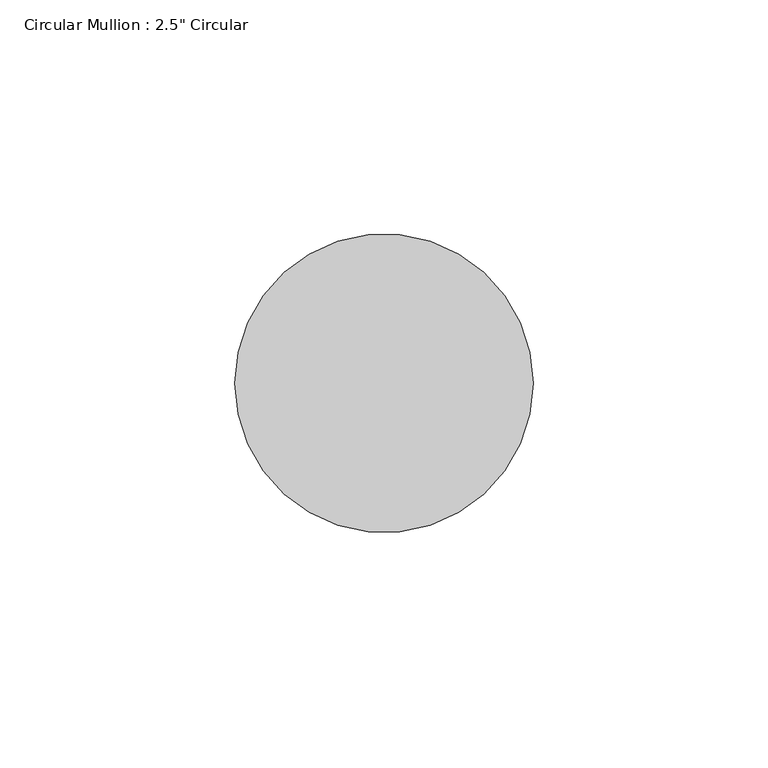
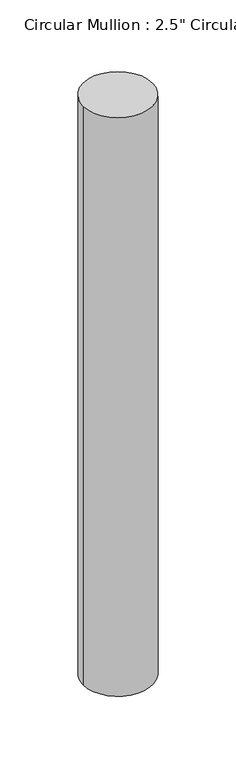
"""IFC4 building model written with IfcOpenShell, lengths in millimetres: member geometry."""

from ifc_helpers import new_model, si_unit, point, frame, origin, origin_2d, place, context, project, spatial, circle_curve, trimmed, segment, composite_curve, outline, extrude, source, transform, mapped, element, save


def member_08c7225e(model_context):
    return source(origin(), model_context, "Body", "SweptSolid", [
        extrude(outline(composite_curve([segment(trimmed(circle_curve(origin_2d(), 31.75), [point((31.75, 0.0))], [point((-31.75, 0.0))], False, "CARTESIAN"), True, "CONTINUOUS"), segment(trimmed(circle_curve(origin_2d(), 31.75), [point((-31.75, 0.0))], [point((31.75, 0.0))], False, "CARTESIAN"), True, "CONTINUOUS")], self_intersect=False)), frame((0.0, 0.0, -558.8), z_axis=(0.0, 0.0, 1.0), x_axis=(1.0, 0.0, 0.0)), (0.0, 0.0, 1.0), 558.8),
    ])


if __name__ == "__main__":
    model = new_model("IFC4")
    model_context = context("Model", 3, world=origin())
    ifc_project = project(units=[si_unit("LENGTHUNIT", "METRE", prefix="MILLI")], contexts=[model_context])
    site = spatial("IfcSite", under=ifc_project)
    building = spatial("IfcBuilding", under=site)
    placement = place(None, origin())
    member_shape = member_08c7225e(model_context)
    element("IfcMember", 1, ObjectType="Circular Mullion : 2.5\" Circular", at=placement, inside=building, context=model_context, shape_type="MappedRepresentation", body=[
        mapped(member_shape, transform((0.0, 0.0, 0.0), x_axis=(1.0, 0.0, 0.0), y_axis=(0.0, 1.0, 0.0), z_axis=(0.0, 0.0, 1.0))),
    ])
    save(model, "model.ifc")

# Revit data of these elements
# Type "Circular Mullion : 2.5\" Circular"
#   built-in parameter 1007350 = 0.104167 (stored number, unit not read)
# Element 1 (IfcMember, "Circular Mullion : 2.5\" Circular")
#   Materials on its faces: "Door - Frame"
# Materials
#   "Door - Frame": colour RGB 118 70 51, transparency 0, Cost = 0
